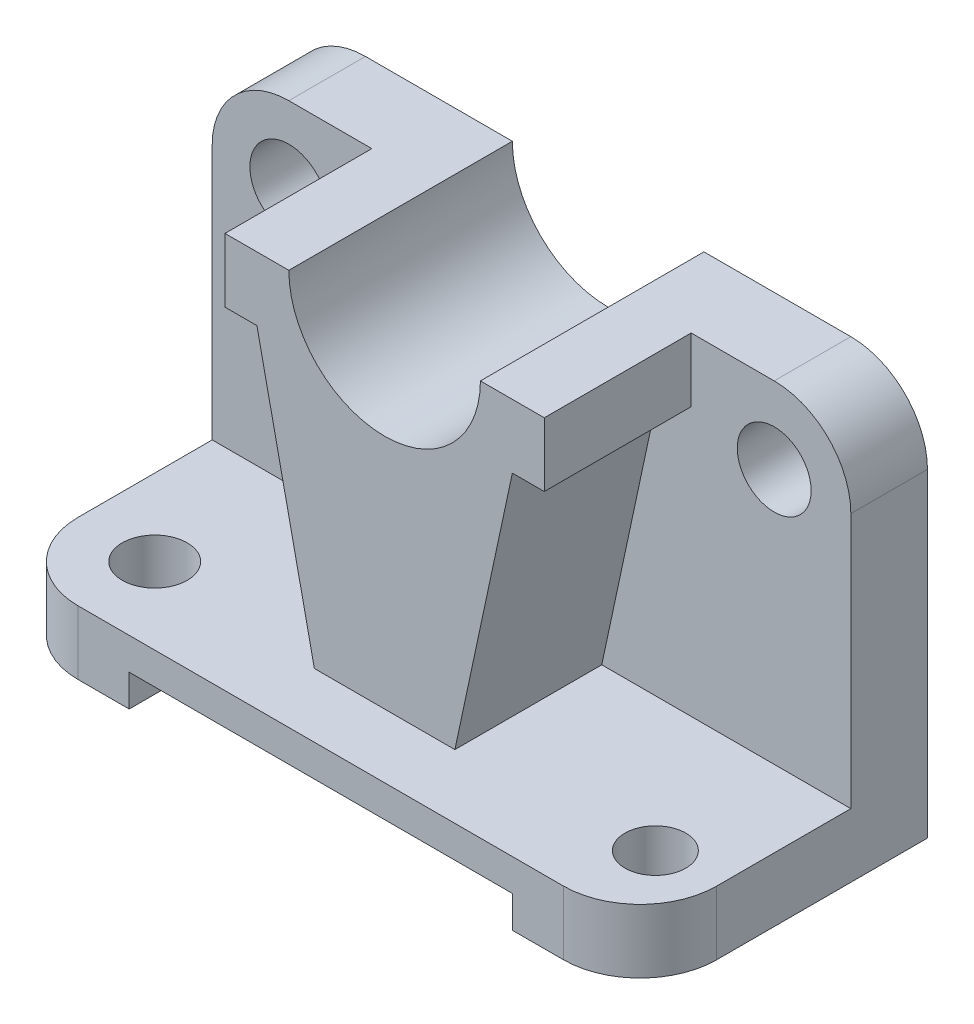
ISO-10303-21;
HEADER;
FILE_DESCRIPTION(('STEP AP214'),'2;1');
FILE_NAME('part.step','',(''),(''),'','','');
FILE_SCHEMA(('AUTOMOTIVE_DESIGN { 1 0 10303 214 1 1 1 1 }'));
ENDSEC;
DATA;
#1=APPLICATION_CONTEXT('core data for automotive mechanical design processes');
#2=APPLICATION_PROTOCOL_DEFINITION('international standard','automotive_design',2000,#1);
#3=PRODUCT_CONTEXT('',#1,'mechanical');
#4=PRODUCT('Part','Part','',(#3));
#5=PRODUCT_RELATED_PRODUCT_CATEGORY('part','',(#4));
#6=PRODUCT_DEFINITION_FORMATION('','',#4);
#7=PRODUCT_DEFINITION_CONTEXT('part definition',#1,'design');
#8=PRODUCT_DEFINITION('design','',#6,#7);
#9=PRODUCT_DEFINITION_SHAPE('','',#8);
#10=(LENGTH_UNIT() NAMED_UNIT(*) SI_UNIT(.MILLI.,.METRE.));
#11=(NAMED_UNIT(*) PLANE_ANGLE_UNIT() SI_UNIT($,.RADIAN.));
#12=(NAMED_UNIT(*) SI_UNIT($,.STERADIAN.) SOLID_ANGLE_UNIT());
#13=UNCERTAINTY_MEASURE_WITH_UNIT(LENGTH_MEASURE(1.E-05),#10,'distance_accuracy_value','');
#14=(GEOMETRIC_REPRESENTATION_CONTEXT(3) GLOBAL_UNCERTAINTY_ASSIGNED_CONTEXT((#13)) GLOBAL_UNIT_ASSIGNED_CONTEXT((#10,
#11,#12)) REPRESENTATION_CONTEXT('',''));
#15=CARTESIAN_POINT('',(0.,0.,0.));
#16=DIRECTION('',(0.,0.,1.));
#17=DIRECTION('',(1.,0.,0.));
#18=AXIS2_PLACEMENT_3D('',#15,#16,#17);
#19=CARTESIAN_POINT('',(0.,62.,-10.5));
#20=DIRECTION('',(0.,-1.,0.));
#21=DIRECTION('',(0.,0.,-1.));
#22=AXIS2_PLACEMENT_3D('',#19,#20,#21);
#23=PLANE('',#22);
#24=DIRECTION('',(1.,0.,0.));
#25=VECTOR('',#24,1.);
#26=CARTESIAN_POINT('',(0.,62.,-10.5));
#27=LINE('',#26,#25);
#28=CARTESIAN_POINT('',(75.,62.,-10.5));
#29=VERTEX_POINT('',#28);
#30=CARTESIAN_POINT('',(88.,62.,-10.5));
#31=VERTEX_POINT('',#30);
#32=EDGE_CURVE('E230',#29,#31,#27,.T.);
#33=ORIENTED_EDGE('',*,*,#32,.T.);
#34=DIRECTION('',(0.,0.,-1.));
#35=VECTOR('',#34,1.);
#36=CARTESIAN_POINT('',(88.,62.,-10.5));
#37=LINE('',#36,#35);
#38=CARTESIAN_POINT('',(88.,62.,-22.5));
#39=VERTEX_POINT('',#38);
#40=EDGE_CURVE('E50',#31,#39,#37,.T.);
#41=ORIENTED_EDGE('',*,*,#40,.T.);
#42=DIRECTION('',(1.,0.,0.));
#43=VECTOR('',#42,1.);
#44=CARTESIAN_POINT('',(0.,62.,-22.5));
#45=LINE('',#44,#43);
#46=CARTESIAN_POINT('',(65.,62.,-22.5));
#47=VERTEX_POINT('',#46);
#48=EDGE_CURVE('E217',#47,#39,#45,.T.);
#49=ORIENTED_EDGE('',*,*,#48,.F.);
#50=DIRECTION('',(0.,0.,-1.));
#51=VECTOR('',#50,1.);
#52=CARTESIAN_POINT('',(65.,62.,12.5));
#53=LINE('',#52,#51);
#54=CARTESIAN_POINT('',(65.,62.,12.5));
#55=VERTEX_POINT('',#54);
#56=EDGE_CURVE('E205',#55,#47,#53,.T.);
#57=ORIENTED_EDGE('',*,*,#56,.F.);
#58=DIRECTION('',(-1.,0.,0.));
#59=VECTOR('',#58,1.);
#60=CARTESIAN_POINT('',(75.,62.,12.5));
#61=LINE('',#60,#59);
#62=CARTESIAN_POINT('',(75.,62.,12.5));
#63=VERTEX_POINT('',#62);
#64=EDGE_CURVE('E456',#63,#55,#61,.T.);
#65=ORIENTED_EDGE('',*,*,#64,.F.);
#66=DIRECTION('',(0.,0.,-1.));
#67=VECTOR('',#66,1.);
#68=CARTESIAN_POINT('',(75.,62.,12.5));
#69=LINE('',#68,#67);
#70=EDGE_CURVE('E211',#63,#29,#69,.T.);
#71=ORIENTED_EDGE('',*,*,#70,.T.);
#72=EDGE_LOOP('',(#33,#41,#49,#57,#65,#71));
#73=FACE_BOUND('',#72,.T.);
#74=ADVANCED_FACE('F39',(#73),#23,.F.);
#75=CARTESIAN_POINT('',(100.,10.,22.5));
#76=DIRECTION('',(0.,-1.,0.));
#77=DIRECTION('',(0.,0.,-1.));
#78=AXIS2_PLACEMENT_3D('',#75,#76,#77);
#79=PLANE('',#78);
#80=CARTESIAN_POINT('',(12.,10.,10.5));
#81=DIRECTION('',(0.,1.,0.));
#82=DIRECTION('',(0.,0.,1.));
#83=AXIS2_PLACEMENT_3D('',#80,#81,#82);
#84=CIRCLE('',#83,5.09061435259613);
#85=CARTESIAN_POINT('',(12.,10.,15.5906143525961));
#86=VERTEX_POINT('',#85);
#87=EDGE_CURVE('E759',#86,#86,#84,.T.);
#88=ORIENTED_EDGE('',*,*,#87,.F.);
#89=EDGE_LOOP('',(#88));
#90=FACE_BOUND('',#89,.T.);
#91=CARTESIAN_POINT('',(90.3964880883435,10.,10.5));
#92=DIRECTION('',(0.,1.,0.));
#93=DIRECTION('',(0.,0.,1.));
#94=AXIS2_PLACEMENT_3D('',#91,#92,#93);
#95=CIRCLE('',#94,4.76218762017058);
#96=CARTESIAN_POINT('',(90.3964880883435,10.,15.2621876201706));
#97=VERTEX_POINT('',#96);
#98=EDGE_CURVE('E762',#97,#97,#95,.T.);
#99=ORIENTED_EDGE('',*,*,#98,.F.);
#100=EDGE_LOOP('',(#99));
#101=FACE_BOUND('',#100,.T.);
#102=DIRECTION('',(0.,0.,-1.));
#103=VECTOR('',#102,1.);
#104=CARTESIAN_POINT('',(0.,10.,22.5));
#105=LINE('',#104,#103);
#106=CARTESIAN_POINT('',(0.,10.,10.5));
#107=VERTEX_POINT('',#106);
#108=CARTESIAN_POINT('',(0.,10.,-10.5));
#109=VERTEX_POINT('',#108);
#110=EDGE_CURVE('E286',#107,#109,#105,.T.);
#111=ORIENTED_EDGE('',*,*,#110,.F.);
#112=CARTESIAN_POINT('',(12.,10.,10.5));
#113=DIRECTION('',(0.,-1.,0.));
#114=DIRECTION('',(0.,0.,-1.));
#115=AXIS2_PLACEMENT_3D('',#112,#113,#114);
#116=CIRCLE('',#115,12.);
#117=CARTESIAN_POINT('',(12.,10.,22.5));
#118=VERTEX_POINT('',#117);
#119=EDGE_CURVE('E308',#107,#118,#116,.F.);
#120=ORIENTED_EDGE('',*,*,#119,.T.);
#121=DIRECTION('',(-1.,0.,0.));
#122=VECTOR('',#121,1.);
#123=CARTESIAN_POINT('',(100.,10.,22.5));
#124=LINE('',#123,#122);
#125=CARTESIAN_POINT('',(88.,10.,22.5));
#126=VERTEX_POINT('',#125);
#127=EDGE_CURVE('E242',#126,#118,#124,.T.);
#128=ORIENTED_EDGE('',*,*,#127,.F.);
#129=CARTESIAN_POINT('',(88.,10.,10.5));
#130=DIRECTION('',(0.,-1.,0.));
#131=DIRECTION('',(0.,0.,-1.));
#132=AXIS2_PLACEMENT_3D('',#129,#130,#131);
#133=CIRCLE('',#132,12.);
#134=CARTESIAN_POINT('',(100.,10.,10.5));
#135=VERTEX_POINT('',#134);
#136=EDGE_CURVE('E303',#126,#135,#133,.F.);
#137=ORIENTED_EDGE('',*,*,#136,.T.);
#138=DIRECTION('',(0.,0.,-1.));
#139=VECTOR('',#138,1.);
#140=CARTESIAN_POINT('',(100.,10.,22.5));
#141=LINE('',#140,#139);
#142=CARTESIAN_POINT('',(100.,10.,-10.5));
#143=VERTEX_POINT('',#142);
#144=EDGE_CURVE('E288',#135,#143,#141,.T.);
#145=ORIENTED_EDGE('',*,*,#144,.T.);
#146=DIRECTION('',(1.,0.,0.));
#147=VECTOR('',#146,1.);
#148=CARTESIAN_POINT('',(0.,10.,-10.5));
#149=LINE('',#148,#147);
#150=CARTESIAN_POINT('',(61.,10.,-10.5));
#151=VERTEX_POINT('',#150);
#152=EDGE_CURVE('E237',#151,#143,#149,.T.);
#153=ORIENTED_EDGE('',*,*,#152,.F.);
#154=DIRECTION('',(0.,0.,-1.));
#155=VECTOR('',#154,1.);
#156=CARTESIAN_POINT('',(61.,10.,12.5));
#157=LINE('',#156,#155);
#158=CARTESIAN_POINT('',(61.,10.,12.5));
#159=VERTEX_POINT('',#158);
#160=EDGE_CURVE('E355',#159,#151,#157,.T.);
#161=ORIENTED_EDGE('',*,*,#160,.F.);
#162=DIRECTION('',(1.,0.,0.));
#163=VECTOR('',#162,1.);
#164=CARTESIAN_POINT('',(39.,10.,12.5));
#165=LINE('',#164,#163);
#166=CARTESIAN_POINT('',(39.,10.,12.5));
#167=VERTEX_POINT('',#166);
#168=EDGE_CURVE('E408',#167,#159,#165,.T.);
#169=ORIENTED_EDGE('',*,*,#168,.F.);
#170=DIRECTION('',(0.,0.,-1.));
#171=VECTOR('',#170,1.);
#172=CARTESIAN_POINT('',(39.,10.,12.5));
#173=LINE('',#172,#171);
#174=CARTESIAN_POINT('',(39.,10.,-10.5));
#175=VERTEX_POINT('',#174);
#176=EDGE_CURVE('E353',#167,#175,#173,.T.);
#177=ORIENTED_EDGE('',*,*,#176,.T.);
#178=EDGE_CURVE('E240',#109,#175,#149,.T.);
#179=ORIENTED_EDGE('',*,*,#178,.F.);
#180=EDGE_LOOP('',(#111,#120,#128,#137,#145,#153,#161,#169,#177,#179));
#181=FACE_BOUND('',#180,.T.);
#182=ADVANCED_FACE('F401',(#90,#101,#181),#79,.F.);
#183=CARTESIAN_POINT('',(0.,10.,-10.5));
#184=DIRECTION('',(0.,0.,-1.));
#185=DIRECTION('',(-1.,0.,0.));
#186=AXIS2_PLACEMENT_3D('',#183,#184,#185);
#187=PLANE('',#186);
#188=CARTESIAN_POINT('',(88.,50.,-10.5));
#189=DIRECTION('',(0.,0.,1.));
#190=DIRECTION('',(1.,0.,0.));
#191=AXIS2_PLACEMENT_3D('',#188,#189,#190);
#192=CIRCLE('',#191,5.78308621894568);
#193=CARTESIAN_POINT('',(93.7830862189457,50.,-10.5));
#194=VERTEX_POINT('',#193);
#195=EDGE_CURVE('E750',#194,#194,#192,.T.);
#196=ORIENTED_EDGE('',*,*,#195,.F.);
#197=EDGE_LOOP('',(#196));
#198=FACE_BOUND('',#197,.T.);
#199=DIRECTION('',(0.,1.,0.));
#200=VECTOR('',#199,1.);
#201=CARTESIAN_POINT('',(100.,10.,-10.5));
#202=LINE('',#201,#200);
#203=CARTESIAN_POINT('',(100.,50.,-10.5));
#204=VERTEX_POINT('',#203);
#205=EDGE_CURVE('E228',#143,#204,#202,.T.);
#206=ORIENTED_EDGE('',*,*,#205,.T.);
#207=CARTESIAN_POINT('',(88.,50.,-10.5));
#208=DIRECTION('',(0.,0.,-1.));
#209=DIRECTION('',(-1.,0.,0.));
#210=AXIS2_PLACEMENT_3D('',#207,#208,#209);
#211=CIRCLE('',#210,12.);
#212=EDGE_CURVE('E11',#204,#31,#211,.F.);
#213=ORIENTED_EDGE('',*,*,#212,.T.);
#214=ORIENTED_EDGE('',*,*,#32,.F.);
#215=DIRECTION('',(0.,1.,0.));
#216=VECTOR('',#215,1.);
#217=CARTESIAN_POINT('',(75.,52.,-10.5));
#218=LINE('',#217,#216);
#219=CARTESIAN_POINT('',(75.,52.,-10.5));
#220=VERTEX_POINT('',#219);
#221=EDGE_CURVE('E423',#220,#29,#218,.T.);
#222=ORIENTED_EDGE('',*,*,#221,.F.);
#223=DIRECTION('',(1.,0.,0.));
#224=VECTOR('',#223,1.);
#225=CARTESIAN_POINT('',(75.,52.,-10.5));
#226=LINE('',#225,#224);
#227=CARTESIAN_POINT('',(70.,52.,-10.5));
#228=VERTEX_POINT('',#227);
#229=EDGE_CURVE('E420',#228,#220,#226,.T.);
#230=ORIENTED_EDGE('',*,*,#229,.F.);
#231=DIRECTION('',(0.209529088730874,0.97780241407741,0.));
#232=VECTOR('',#231,1.);
#233=CARTESIAN_POINT('',(70.,52.,-10.5));
#234=LINE('',#233,#232);
#235=EDGE_CURVE('E412',#151,#228,#234,.T.);
#236=ORIENTED_EDGE('',*,*,#235,.F.);
#237=ORIENTED_EDGE('',*,*,#152,.T.);
#238=EDGE_LOOP('',(#206,#213,#214,#222,#230,#236,#237));
#239=FACE_BOUND('',#238,.T.);
#240=ADVANCED_FACE('F362',(#198,#239),#187,.F.);
#241=CARTESIAN_POINT('',(12.,50.,-10.5));
#242=DIRECTION('',(0.,0.,1.));
#243=DIRECTION('',(1.,0.,0.));
#244=AXIS2_PLACEMENT_3D('',#241,#242,#243);
#245=CIRCLE('',#244,6.102513624206);
#246=CARTESIAN_POINT('',(18.102513624206,50.,-10.5));
#247=VERTEX_POINT('',#246);
#248=EDGE_CURVE('E225',#247,#247,#245,.T.);
#249=ORIENTED_EDGE('',*,*,#248,.F.);
#250=EDGE_LOOP('',(#249));
#251=FACE_BOUND('',#250,.T.);
#252=CARTESIAN_POINT('',(12.,62.,-10.5));
#253=VERTEX_POINT('',#252);
#254=CARTESIAN_POINT('',(25.,62.,-10.5));
#255=VERTEX_POINT('',#254);
#256=EDGE_CURVE('E233',#253,#255,#27,.T.);
#257=ORIENTED_EDGE('',*,*,#256,.F.);
#258=CARTESIAN_POINT('',(12.,50.,-10.5));
#259=DIRECTION('',(0.,0.,-1.));
#260=DIRECTION('',(-1.,0.,0.));
#261=AXIS2_PLACEMENT_3D('',#258,#259,#260);
#262=CIRCLE('',#261,12.);
#263=CARTESIAN_POINT('',(0.,50.,-10.5));
#264=VERTEX_POINT('',#263);
#265=EDGE_CURVE('E317',#253,#264,#262,.F.);
#266=ORIENTED_EDGE('',*,*,#265,.T.);
#267=DIRECTION('',(0.,1.,0.));
#268=VECTOR('',#267,1.);
#269=CARTESIAN_POINT('',(0.,10.,-10.5));
#270=LINE('',#269,#268);
#271=EDGE_CURVE('E227',#109,#264,#270,.T.);
#272=ORIENTED_EDGE('',*,*,#271,.F.);
#273=ORIENTED_EDGE('',*,*,#178,.T.);
#274=DIRECTION('',(0.209529088730874,-0.977802414077409,0.));
#275=VECTOR('',#274,1.);
#276=CARTESIAN_POINT('',(30.,52.,-10.5));
#277=LINE('',#276,#275);
#278=CARTESIAN_POINT('',(30.,52.,-10.5));
#279=VERTEX_POINT('',#278);
#280=EDGE_CURVE('E222',#279,#175,#277,.T.);
#281=ORIENTED_EDGE('',*,*,#280,.F.);
#282=DIRECTION('',(1.,0.,0.));
#283=VECTOR('',#282,1.);
#284=CARTESIAN_POINT('',(25.,52.,-10.5));
#285=LINE('',#284,#283);
#286=CARTESIAN_POINT('',(25.,52.,-10.5));
#287=VERTEX_POINT('',#286);
#288=EDGE_CURVE('E427',#287,#279,#285,.T.);
#289=ORIENTED_EDGE('',*,*,#288,.F.);
#290=DIRECTION('',(0.,-1.,0.));
#291=VECTOR('',#290,1.);
#292=CARTESIAN_POINT('',(25.,62.,-10.5));
#293=LINE('',#292,#291);
#294=EDGE_CURVE('E430',#255,#287,#293,.T.);
#295=ORIENTED_EDGE('',*,*,#294,.F.);
#296=EDGE_LOOP('',(#257,#266,#272,#273,#281,#289,#295));
#297=FACE_BOUND('',#296,.T.);
#298=ADVANCED_FACE('F323',(#251,#297),#187,.F.);
#299=CARTESIAN_POINT('',(100.,0.,22.5));
#300=DIRECTION('',(-1.,0.,0.));
#301=DIRECTION('',(0.,0.,1.));
#302=AXIS2_PLACEMENT_3D('',#299,#300,#301);
#303=PLANE('',#302);
#304=ORIENTED_EDGE('',*,*,#144,.F.);
#305=DIRECTION('',(0.,1.,0.));
#306=VECTOR('',#305,1.);
#307=CARTESIAN_POINT('',(100.,0.,10.5));
#308=LINE('',#307,#306);
#309=CARTESIAN_POINT('',(100.,0.,10.5));
#310=VERTEX_POINT('',#309);
#311=EDGE_CURVE('E309',#135,#310,#308,.F.);
#312=ORIENTED_EDGE('',*,*,#311,.T.);
#313=DIRECTION('',(0.,0.,-1.));
#314=VECTOR('',#313,1.);
#315=CARTESIAN_POINT('',(100.,0.,22.5));
#316=LINE('',#315,#314);
#317=CARTESIAN_POINT('',(100.,0.,-22.5));
#318=VERTEX_POINT('',#317);
#319=EDGE_CURVE('E258',#310,#318,#316,.T.);
#320=ORIENTED_EDGE('',*,*,#319,.T.);
#321=DIRECTION('',(0.,1.,0.));
#322=VECTOR('',#321,1.);
#323=CARTESIAN_POINT('',(100.,0.,-22.5));
#324=LINE('',#323,#322);
#325=CARTESIAN_POINT('',(100.,50.,-22.5));
#326=VERTEX_POINT('',#325);
#327=EDGE_CURVE('E238',#318,#326,#324,.T.);
#328=ORIENTED_EDGE('',*,*,#327,.T.);
#329=DIRECTION('',(0.,0.,-1.));
#330=VECTOR('',#329,1.);
#331=CARTESIAN_POINT('',(100.,50.,22.5));
#332=LINE('',#331,#330);
#333=EDGE_CURVE('E306',#326,#204,#332,.F.);
#334=ORIENTED_EDGE('',*,*,#333,.T.);
#335=ORIENTED_EDGE('',*,*,#205,.F.);
#336=EDGE_LOOP('',(#304,#312,#320,#328,#334,#335));
#337=FACE_BOUND('',#336,.T.);
#338=ADVANCED_FACE('F371',(#337),#303,.F.);
#339=CARTESIAN_POINT('',(0.,10.,22.5));
#340=DIRECTION('',(1.,0.,0.));
#341=DIRECTION('',(0.,0.,-1.));
#342=AXIS2_PLACEMENT_3D('',#339,#340,#341);
#343=PLANE('',#342);
#344=DIRECTION('',(0.,0.,-1.));
#345=VECTOR('',#344,1.);
#346=CARTESIAN_POINT('',(0.,0.,22.5));
#347=LINE('',#346,#345);
#348=CARTESIAN_POINT('',(0.,0.,10.5));
#349=VERTEX_POINT('',#348);
#350=CARTESIAN_POINT('',(0.,0.,-22.5));
#351=VERTEX_POINT('',#350);
#352=EDGE_CURVE('E281',#349,#351,#347,.T.);
#353=ORIENTED_EDGE('',*,*,#352,.F.);
#354=DIRECTION('',(0.,-1.,0.));
#355=VECTOR('',#354,1.);
#356=CARTESIAN_POINT('',(0.,10.,10.5));
#357=LINE('',#356,#355);
#358=EDGE_CURVE('E301',#349,#107,#357,.F.);
#359=ORIENTED_EDGE('',*,*,#358,.T.);
#360=ORIENTED_EDGE('',*,*,#110,.T.);
#361=ORIENTED_EDGE('',*,*,#271,.T.);
#362=DIRECTION('',(0.,0.,-1.));
#363=VECTOR('',#362,1.);
#364=CARTESIAN_POINT('',(0.,50.,22.5));
#365=LINE('',#364,#363);
#366=CARTESIAN_POINT('',(0.,50.,-22.5));
#367=VERTEX_POINT('',#366);
#368=EDGE_CURVE('E296',#264,#367,#365,.T.);
#369=ORIENTED_EDGE('',*,*,#368,.T.);
#370=DIRECTION('',(0.,-1.,0.));
#371=VECTOR('',#370,1.);
#372=CARTESIAN_POINT('',(0.,10.,-22.5));
#373=LINE('',#372,#371);
#374=EDGE_CURVE('E259',#367,#351,#373,.T.);
#375=ORIENTED_EDGE('',*,*,#374,.T.);
#376=EDGE_LOOP('',(#353,#359,#360,#361,#369,#375));
#377=FACE_BOUND('',#376,.T.);
#378=ADVANCED_FACE('F328',(#377),#343,.F.);
#379=CARTESIAN_POINT('',(0.,0.,22.5));
#380=DIRECTION('',(0.,1.,0.));
#381=DIRECTION('',(0.,0.,1.));
#382=AXIS2_PLACEMENT_3D('',#379,#380,#381);
#383=PLANE('',#382);
#384=CARTESIAN_POINT('',(12.,0.,10.5));
#385=DIRECTION('',(0.,1.,0.));
#386=DIRECTION('',(0.,0.,1.));
#387=AXIS2_PLACEMENT_3D('',#384,#385,#386);
#388=CIRCLE('',#387,5.09061435259613);
#389=CARTESIAN_POINT('',(12.,0.,15.5906143525961));
#390=VERTEX_POINT('',#389);
#391=EDGE_CURVE('E760',#390,#390,#388,.T.);
#392=ORIENTED_EDGE('',*,*,#391,.T.);
#393=EDGE_LOOP('',(#392));
#394=FACE_BOUND('',#393,.T.);
#395=DIRECTION('',(1.,0.,0.));
#396=VECTOR('',#395,1.);
#397=CARTESIAN_POINT('',(0.,0.,22.5));
#398=LINE('',#397,#396);
#399=CARTESIAN_POINT('',(12.,0.,22.5));
#400=VERTEX_POINT('',#399);
#401=CARTESIAN_POINT('',(20.,0.,22.5));
#402=VERTEX_POINT('',#401);
#403=EDGE_CURVE('E241',#400,#402,#398,.T.);
#404=ORIENTED_EDGE('',*,*,#403,.F.);
#405=CARTESIAN_POINT('',(12.,0.,10.5));
#406=DIRECTION('',(0.,1.,0.));
#407=DIRECTION('',(0.,0.,1.));
#408=AXIS2_PLACEMENT_3D('',#405,#406,#407);
#409=CIRCLE('',#408,12.);
#410=EDGE_CURVE('E299',#400,#349,#409,.F.);
#411=ORIENTED_EDGE('',*,*,#410,.T.);
#412=ORIENTED_EDGE('',*,*,#352,.T.);
#413=DIRECTION('',(1.,0.,0.));
#414=VECTOR('',#413,1.);
#415=CARTESIAN_POINT('',(0.,0.,-22.5));
#416=LINE('',#415,#414);
#417=CARTESIAN_POINT('',(20.,0.,-22.5));
#418=VERTEX_POINT('',#417);
#419=EDGE_CURVE('E261',#351,#418,#416,.T.);
#420=ORIENTED_EDGE('',*,*,#419,.T.);
#421=DIRECTION('',(0.,0.,-1.));
#422=VECTOR('',#421,1.);
#423=CARTESIAN_POINT('',(20.,0.,22.5));
#424=LINE('',#423,#422);
#425=EDGE_CURVE('E282',#402,#418,#424,.T.);
#426=ORIENTED_EDGE('',*,*,#425,.F.);
#427=EDGE_LOOP('',(#404,#411,#412,#420,#426));
#428=FACE_BOUND('',#427,.T.);
#429=ADVANCED_FACE('F399',(#394,#428),#383,.F.);
#430=CARTESIAN_POINT('',(20.,0.,22.5));
#431=DIRECTION('',(-1.,0.,0.));
#432=DIRECTION('',(0.,0.,1.));
#433=AXIS2_PLACEMENT_3D('',#430,#431,#432);
#434=PLANE('',#433);
#435=DIRECTION('',(0.,1.,0.));
#436=VECTOR('',#435,1.);
#437=CARTESIAN_POINT('',(20.,0.,-22.5));
#438=LINE('',#437,#436);
#439=CARTESIAN_POINT('',(20.,5.,-22.5));
#440=VERTEX_POINT('',#439);
#441=EDGE_CURVE('E263',#418,#440,#438,.T.);
#442=ORIENTED_EDGE('',*,*,#441,.T.);
#443=DIRECTION('',(0.,0.,-1.));
#444=VECTOR('',#443,1.);
#445=CARTESIAN_POINT('',(20.,5.,22.5));
#446=LINE('',#445,#444);
#447=CARTESIAN_POINT('',(20.,5.,22.5));
#448=VERTEX_POINT('',#447);
#449=EDGE_CURVE('E279',#448,#440,#446,.T.);
#450=ORIENTED_EDGE('',*,*,#449,.F.);
#451=DIRECTION('',(0.,1.,0.));
#452=VECTOR('',#451,1.);
#453=CARTESIAN_POINT('',(20.,0.,22.5));
#454=LINE('',#453,#452);
#455=EDGE_CURVE('E246',#402,#448,#454,.T.);
#456=ORIENTED_EDGE('',*,*,#455,.F.);
#457=ORIENTED_EDGE('',*,*,#425,.T.);
#458=EDGE_LOOP('',(#442,#450,#456,#457));
#459=FACE_BOUND('',#458,.T.);
#460=ADVANCED_FACE('F394',(#459),#434,.F.);
#461=CARTESIAN_POINT('',(20.,5.,22.5));
#462=DIRECTION('',(0.,1.,0.));
#463=DIRECTION('',(0.,0.,1.));
#464=AXIS2_PLACEMENT_3D('',#461,#462,#463);
#465=PLANE('',#464);
#466=DIRECTION('',(1.,0.,0.));
#467=VECTOR('',#466,1.);
#468=CARTESIAN_POINT('',(20.,5.,-22.5));
#469=LINE('',#468,#467);
#470=CARTESIAN_POINT('',(80.,5.,-22.5));
#471=VERTEX_POINT('',#470);
#472=EDGE_CURVE('E264',#440,#471,#469,.T.);
#473=ORIENTED_EDGE('',*,*,#472,.T.);
#474=DIRECTION('',(0.,0.,-1.));
#475=VECTOR('',#474,1.);
#476=CARTESIAN_POINT('',(80.,5.,22.5));
#477=LINE('',#476,#475);
#478=CARTESIAN_POINT('',(80.,5.,22.5));
#479=VERTEX_POINT('',#478);
#480=EDGE_CURVE('E274',#479,#471,#477,.T.);
#481=ORIENTED_EDGE('',*,*,#480,.F.);
#482=DIRECTION('',(1.,0.,0.));
#483=VECTOR('',#482,1.);
#484=CARTESIAN_POINT('',(20.,5.,22.5));
#485=LINE('',#484,#483);
#486=EDGE_CURVE('E248',#448,#479,#485,.T.);
#487=ORIENTED_EDGE('',*,*,#486,.F.);
#488=ORIENTED_EDGE('',*,*,#449,.T.);
#489=EDGE_LOOP('',(#473,#481,#487,#488));
#490=FACE_BOUND('',#489,.T.);
#491=ADVANCED_FACE('F389',(#490),#465,.F.);
#492=CARTESIAN_POINT('',(80.,5.,22.5));
#493=DIRECTION('',(1.,0.,0.));
#494=DIRECTION('',(0.,0.,-1.));
#495=AXIS2_PLACEMENT_3D('',#492,#493,#494);
#496=PLANE('',#495);
#497=DIRECTION('',(0.,-1.,0.));
#498=VECTOR('',#497,1.);
#499=CARTESIAN_POINT('',(80.,5.,-22.5));
#500=LINE('',#499,#498);
#501=CARTESIAN_POINT('',(80.,0.,-22.5));
#502=VERTEX_POINT('',#501);
#503=EDGE_CURVE('E270',#471,#502,#500,.T.);
#504=ORIENTED_EDGE('',*,*,#503,.T.);
#505=DIRECTION('',(0.,0.,-1.));
#506=VECTOR('',#505,1.);
#507=CARTESIAN_POINT('',(80.,0.,22.5));
#508=LINE('',#507,#506);
#509=CARTESIAN_POINT('',(80.,0.,22.5));
#510=VERTEX_POINT('',#509);
#511=EDGE_CURVE('E275',#510,#502,#508,.T.);
#512=ORIENTED_EDGE('',*,*,#511,.F.);
#513=DIRECTION('',(0.,-1.,0.));
#514=VECTOR('',#513,1.);
#515=CARTESIAN_POINT('',(80.,5.,22.5));
#516=LINE('',#515,#514);
#517=EDGE_CURVE('E253',#479,#510,#516,.T.);
#518=ORIENTED_EDGE('',*,*,#517,.F.);
#519=ORIENTED_EDGE('',*,*,#480,.T.);
#520=EDGE_LOOP('',(#504,#512,#518,#519));
#521=FACE_BOUND('',#520,.T.);
#522=ADVANCED_FACE('F382',(#521),#496,.F.);
#523=CARTESIAN_POINT('',(80.,0.,22.5));
#524=DIRECTION('',(0.,1.,0.));
#525=DIRECTION('',(0.,0.,1.));
#526=AXIS2_PLACEMENT_3D('',#523,#524,#525);
#527=PLANE('',#526);
#528=CARTESIAN_POINT('',(90.3964880883435,0.,10.5));
#529=DIRECTION('',(0.,1.,0.));
#530=DIRECTION('',(0.,0.,1.));
#531=AXIS2_PLACEMENT_3D('',#528,#529,#530);
#532=CIRCLE('',#531,4.76218762017058);
#533=CARTESIAN_POINT('',(90.3964880883435,0.,15.2621876201706));
#534=VERTEX_POINT('',#533);
#535=EDGE_CURVE('E755',#534,#534,#532,.T.);
#536=ORIENTED_EDGE('',*,*,#535,.T.);
#537=EDGE_LOOP('',(#536));
#538=FACE_BOUND('',#537,.T.);
#539=ORIENTED_EDGE('',*,*,#319,.F.);
#540=CARTESIAN_POINT('',(88.,0.,10.5));
#541=DIRECTION('',(0.,1.,0.));
#542=DIRECTION('',(0.,0.,1.));
#543=AXIS2_PLACEMENT_3D('',#540,#541,#542);
#544=CIRCLE('',#543,12.);
#545=CARTESIAN_POINT('',(88.,0.,22.5));
#546=VERTEX_POINT('',#545);
#547=EDGE_CURVE('E315',#310,#546,#544,.F.);
#548=ORIENTED_EDGE('',*,*,#547,.T.);
#549=DIRECTION('',(1.,0.,0.));
#550=VECTOR('',#549,1.);
#551=CARTESIAN_POINT('',(80.,0.,22.5));
#552=LINE('',#551,#550);
#553=EDGE_CURVE('E251',#510,#546,#552,.T.);
#554=ORIENTED_EDGE('',*,*,#553,.F.);
#555=ORIENTED_EDGE('',*,*,#511,.T.);
#556=DIRECTION('',(1.,0.,0.));
#557=VECTOR('',#556,1.);
#558=CARTESIAN_POINT('',(80.,0.,-22.5));
#559=LINE('',#558,#557);
#560=EDGE_CURVE('E243',#502,#318,#559,.T.);
#561=ORIENTED_EDGE('',*,*,#560,.T.);
#562=EDGE_LOOP('',(#539,#548,#554,#555,#561));
#563=FACE_BOUND('',#562,.T.);
#564=ADVANCED_FACE('F376',(#538,#563),#527,.F.);
#565=CARTESIAN_POINT('',(0.,0.,22.5));
#566=DIRECTION('',(0.,0.,1.));
#567=DIRECTION('',(1.,0.,0.));
#568=AXIS2_PLACEMENT_3D('',#565,#566,#567);
#569=PLANE('',#568);
#570=ORIENTED_EDGE('',*,*,#127,.T.);
#571=DIRECTION('',(0.,-1.,0.));
#572=VECTOR('',#571,1.);
#573=CARTESIAN_POINT('',(12.,0.,22.5));
#574=LINE('',#573,#572);
#575=EDGE_CURVE('E294',#118,#400,#574,.T.);
#576=ORIENTED_EDGE('',*,*,#575,.T.);
#577=ORIENTED_EDGE('',*,*,#403,.T.);
#578=ORIENTED_EDGE('',*,*,#455,.T.);
#579=ORIENTED_EDGE('',*,*,#486,.T.);
#580=ORIENTED_EDGE('',*,*,#517,.T.);
#581=ORIENTED_EDGE('',*,*,#553,.T.);
#582=DIRECTION('',(0.,1.,0.));
#583=VECTOR('',#582,1.);
#584=CARTESIAN_POINT('',(88.,10.,22.5));
#585=LINE('',#584,#583);
#586=EDGE_CURVE('E292',#546,#126,#585,.T.);
#587=ORIENTED_EDGE('',*,*,#586,.T.);
#588=EDGE_LOOP('',(#570,#576,#577,#578,#579,#580,#581,#587));
#589=FACE_BOUND('',#588,.T.);
#590=ADVANCED_FACE('F403',(#589),#569,.T.);
#591=CARTESIAN_POINT('',(0.,0.,-22.5));
#592=DIRECTION('',(0.,0.,1.));
#593=DIRECTION('',(1.,0.,0.));
#594=AXIS2_PLACEMENT_3D('',#591,#592,#593);
#595=PLANE('',#594);
#596=CARTESIAN_POINT('',(88.,50.,-22.5));
#597=DIRECTION('',(0.,0.,1.));
#598=DIRECTION('',(1.,0.,0.));
#599=AXIS2_PLACEMENT_3D('',#596,#597,#598);
#600=CIRCLE('',#599,5.78308621894568);
#601=CARTESIAN_POINT('',(93.7830862189457,50.,-22.5));
#602=VERTEX_POINT('',#601);
#603=EDGE_CURVE('E756',#602,#602,#600,.T.);
#604=ORIENTED_EDGE('',*,*,#603,.T.);
#605=EDGE_LOOP('',(#604));
#606=FACE_BOUND('',#605,.T.);
#607=CARTESIAN_POINT('',(12.,50.,-22.5));
#608=DIRECTION('',(0.,0.,1.));
#609=DIRECTION('',(1.,0.,0.));
#610=AXIS2_PLACEMENT_3D('',#607,#608,#609);
#611=CIRCLE('',#610,6.102513624206);
#612=CARTESIAN_POINT('',(18.102513624206,50.,-22.5));
#613=VERTEX_POINT('',#612);
#614=EDGE_CURVE('E748',#613,#613,#611,.T.);
#615=ORIENTED_EDGE('',*,*,#614,.T.);
#616=EDGE_LOOP('',(#615));
#617=FACE_BOUND('',#616,.T.);
#618=ORIENTED_EDGE('',*,*,#374,.F.);
#619=CARTESIAN_POINT('',(12.,50.,-22.5));
#620=DIRECTION('',(0.,0.,1.));
#621=DIRECTION('',(1.,0.,0.));
#622=AXIS2_PLACEMENT_3D('',#619,#620,#621);
#623=CIRCLE('',#622,12.);
#624=CARTESIAN_POINT('',(12.,62.,-22.5));
#625=VERTEX_POINT('',#624);
#626=EDGE_CURVE('E316',#367,#625,#623,.F.);
#627=ORIENTED_EDGE('',*,*,#626,.T.);
#628=CARTESIAN_POINT('',(35.,62.,-22.5));
#629=VERTEX_POINT('',#628);
#630=EDGE_CURVE('E218',#625,#629,#45,.T.);
#631=ORIENTED_EDGE('',*,*,#630,.T.);
#632=CARTESIAN_POINT('',(50.,62.,-22.5));
#633=DIRECTION('',(0.,0.,1.));
#634=DIRECTION('',(1.,0.,0.));
#635=AXIS2_PLACEMENT_3D('',#632,#633,#634);
#636=CIRCLE('',#635,15.);
#637=EDGE_CURVE('E206',#629,#47,#636,.T.);
#638=ORIENTED_EDGE('',*,*,#637,.T.);
#639=ORIENTED_EDGE('',*,*,#48,.T.);
#640=CARTESIAN_POINT('',(88.,50.,-22.5));
#641=DIRECTION('',(0.,0.,1.));
#642=DIRECTION('',(1.,0.,0.));
#643=AXIS2_PLACEMENT_3D('',#640,#641,#642);
#644=CIRCLE('',#643,12.);
#645=EDGE_CURVE('E314',#39,#326,#644,.F.);
#646=ORIENTED_EDGE('',*,*,#645,.T.);
#647=ORIENTED_EDGE('',*,*,#327,.F.);
#648=ORIENTED_EDGE('',*,*,#560,.F.);
#649=ORIENTED_EDGE('',*,*,#503,.F.);
#650=ORIENTED_EDGE('',*,*,#472,.F.);
#651=ORIENTED_EDGE('',*,*,#441,.F.);
#652=ORIENTED_EDGE('',*,*,#419,.F.);
#653=EDGE_LOOP('',(#618,#627,#631,#638,#639,#646,#647,#648,#649,#650,#651,#652));
#654=FACE_BOUND('',#653,.T.);
#655=ADVANCED_FACE('F220',(#606,#617,#654),#595,.F.);
#656=ORIENTED_EDGE('',*,*,#630,.F.);
#657=DIRECTION('',(0.,0.,-1.));
#658=VECTOR('',#657,1.);
#659=CARTESIAN_POINT('',(12.,62.,-10.5));
#660=LINE('',#659,#658);
#661=EDGE_CURVE('E58',#625,#253,#660,.F.);
#662=ORIENTED_EDGE('',*,*,#661,.T.);
#663=ORIENTED_EDGE('',*,*,#256,.T.);
#664=DIRECTION('',(0.,0.,-1.));
#665=VECTOR('',#664,1.);
#666=CARTESIAN_POINT('',(25.,62.,12.5));
#667=LINE('',#666,#665);
#668=CARTESIAN_POINT('',(25.,62.,12.5));
#669=VERTEX_POINT('',#668);
#670=EDGE_CURVE('E340',#669,#255,#667,.T.);
#671=ORIENTED_EDGE('',*,*,#670,.F.);
#672=DIRECTION('',(-1.,0.,0.));
#673=VECTOR('',#672,1.);
#674=CARTESIAN_POINT('',(35.,62.,12.5));
#675=LINE('',#674,#673);
#676=CARTESIAN_POINT('',(35.,62.,12.5));
#677=VERTEX_POINT('',#676);
#678=EDGE_CURVE('E339',#677,#669,#675,.T.);
#679=ORIENTED_EDGE('',*,*,#678,.F.);
#680=DIRECTION('',(0.,0.,-1.));
#681=VECTOR('',#680,1.);
#682=CARTESIAN_POINT('',(35.,62.,12.5));
#683=LINE('',#682,#681);
#684=EDGE_CURVE('E215',#677,#629,#683,.T.);
#685=ORIENTED_EDGE('',*,*,#684,.T.);
#686=EDGE_LOOP('',(#656,#662,#663,#671,#679,#685));
#687=FACE_BOUND('',#686,.T.);
#688=ADVANCED_FACE('F331',(#687),#23,.F.);
#689=CARTESIAN_POINT('',(30.,52.,12.5));
#690=DIRECTION('',(0.977802414077409,0.209529088730874,0.));
#691=DIRECTION('',(-0.209529088730874,0.977802414077409,0.));
#692=AXIS2_PLACEMENT_3D('',#689,#690,#691);
#693=PLANE('',#692);
#694=ORIENTED_EDGE('',*,*,#280,.T.);
#695=ORIENTED_EDGE('',*,*,#176,.F.);
#696=DIRECTION('',(0.209529088730874,-0.977802414077409,0.));
#697=VECTOR('',#696,1.);
#698=CARTESIAN_POINT('',(30.,52.,12.5));
#699=LINE('',#698,#697);
#700=CARTESIAN_POINT('',(30.,52.,12.5));
#701=VERTEX_POINT('',#700);
#702=EDGE_CURVE('E431',#701,#167,#699,.T.);
#703=ORIENTED_EDGE('',*,*,#702,.F.);
#704=DIRECTION('',(0.,0.,-1.));
#705=VECTOR('',#704,1.);
#706=CARTESIAN_POINT('',(30.,52.,12.5));
#707=LINE('',#706,#705);
#708=EDGE_CURVE('E435',#701,#279,#707,.T.);
#709=ORIENTED_EDGE('',*,*,#708,.T.);
#710=EDGE_LOOP('',(#694,#695,#703,#709));
#711=FACE_BOUND('',#710,.T.);
#712=ADVANCED_FACE('F447',(#711),#693,.F.);
#713=CARTESIAN_POINT('',(70.,52.,12.5));
#714=DIRECTION('',(-0.977802414077409,0.209529088730874,0.));
#715=DIRECTION('',(-0.209529088730874,-0.97780241407741,0.));
#716=AXIS2_PLACEMENT_3D('',#713,#714,#715);
#717=PLANE('',#716);
#718=ORIENTED_EDGE('',*,*,#235,.T.);
#719=DIRECTION('',(0.,0.,-1.));
#720=VECTOR('',#719,1.);
#721=CARTESIAN_POINT('',(70.,52.,12.5));
#722=LINE('',#721,#720);
#723=CARTESIAN_POINT('',(70.,52.,12.5));
#724=VERTEX_POINT('',#723);
#725=EDGE_CURVE('E348',#724,#228,#722,.T.);
#726=ORIENTED_EDGE('',*,*,#725,.F.);
#727=DIRECTION('',(0.209529088730874,0.97780241407741,0.));
#728=VECTOR('',#727,1.);
#729=CARTESIAN_POINT('',(70.,52.,12.5));
#730=LINE('',#729,#728);
#731=EDGE_CURVE('E418',#159,#724,#730,.T.);
#732=ORIENTED_EDGE('',*,*,#731,.F.);
#733=ORIENTED_EDGE('',*,*,#160,.T.);
#734=EDGE_LOOP('',(#718,#726,#732,#733));
#735=FACE_BOUND('',#734,.T.);
#736=ADVANCED_FACE('F415',(#735),#717,.F.);
#737=CARTESIAN_POINT('',(75.,52.,12.5));
#738=DIRECTION('',(0.,1.,0.));
#739=DIRECTION('',(0.,0.,1.));
#740=AXIS2_PLACEMENT_3D('',#737,#738,#739);
#741=PLANE('',#740);
#742=ORIENTED_EDGE('',*,*,#229,.T.);
#743=DIRECTION('',(0.,0.,-1.));
#744=VECTOR('',#743,1.);
#745=CARTESIAN_POINT('',(75.,52.,12.5));
#746=LINE('',#745,#744);
#747=CARTESIAN_POINT('',(75.,52.,12.5));
#748=VERTEX_POINT('',#747);
#749=EDGE_CURVE('E350',#748,#220,#746,.T.);
#750=ORIENTED_EDGE('',*,*,#749,.F.);
#751=DIRECTION('',(1.,0.,0.));
#752=VECTOR('',#751,1.);
#753=CARTESIAN_POINT('',(75.,52.,12.5));
#754=LINE('',#753,#752);
#755=EDGE_CURVE('E453',#724,#748,#754,.T.);
#756=ORIENTED_EDGE('',*,*,#755,.F.);
#757=ORIENTED_EDGE('',*,*,#725,.T.);
#758=EDGE_LOOP('',(#742,#750,#756,#757));
#759=FACE_BOUND('',#758,.T.);
#760=ADVANCED_FACE('F621',(#759),#741,.F.);
#761=CARTESIAN_POINT('',(75.,52.,12.5));
#762=DIRECTION('',(-1.,0.,0.));
#763=DIRECTION('',(0.,0.,1.));
#764=AXIS2_PLACEMENT_3D('',#761,#762,#763);
#765=PLANE('',#764);
#766=ORIENTED_EDGE('',*,*,#221,.T.);
#767=ORIENTED_EDGE('',*,*,#70,.F.);
#768=DIRECTION('',(0.,1.,0.));
#769=VECTOR('',#768,1.);
#770=CARTESIAN_POINT('',(75.,52.,12.5));
#771=LINE('',#770,#769);
#772=EDGE_CURVE('E457',#748,#63,#771,.T.);
#773=ORIENTED_EDGE('',*,*,#772,.F.);
#774=ORIENTED_EDGE('',*,*,#749,.T.);
#775=EDGE_LOOP('',(#766,#767,#773,#774));
#776=FACE_BOUND('',#775,.T.);
#777=ADVANCED_FACE('F471',(#776),#765,.F.);
#778=CARTESIAN_POINT('',(50.,62.,12.5));
#779=DIRECTION('',(0.,0.,-1.));
#780=DIRECTION('',(-1.,0.,0.));
#781=AXIS2_PLACEMENT_3D('',#778,#779,#780);
#782=CYLINDRICAL_SURFACE('',#781,15.);
#783=ORIENTED_EDGE('',*,*,#56,.T.);
#784=ORIENTED_EDGE('',*,*,#637,.F.);
#785=ORIENTED_EDGE('',*,*,#684,.F.);
#786=CARTESIAN_POINT('',(50.,62.,12.5));
#787=DIRECTION('',(0.,0.,-1.));
#788=DIRECTION('',(1.,0.,0.));
#789=AXIS2_PLACEMENT_3D('',#786,#787,#788);
#790=CIRCLE('',#789,15.);
#791=EDGE_CURVE('E210',#55,#677,#790,.T.);
#792=ORIENTED_EDGE('',*,*,#791,.F.);
#793=EDGE_LOOP('',(#783,#784,#785,#792));
#794=FACE_BOUND('',#793,.T.);
#795=ADVANCED_FACE('F204',(#794),#782,.F.);
#796=CARTESIAN_POINT('',(25.,62.,12.5));
#797=DIRECTION('',(1.,0.,0.));
#798=DIRECTION('',(0.,1.,0.));
#799=AXIS2_PLACEMENT_3D('',#796,#797,#798);
#800=PLANE('',#799);
#801=ORIENTED_EDGE('',*,*,#294,.T.);
#802=DIRECTION('',(0.,0.,-1.));
#803=VECTOR('',#802,1.);
#804=CARTESIAN_POINT('',(25.,52.,12.5));
#805=LINE('',#804,#803);
#806=CARTESIAN_POINT('',(25.,52.,12.5));
#807=VERTEX_POINT('',#806);
#808=EDGE_CURVE('E344',#807,#287,#805,.T.);
#809=ORIENTED_EDGE('',*,*,#808,.F.);
#810=DIRECTION('',(0.,-1.,0.));
#811=VECTOR('',#810,1.);
#812=CARTESIAN_POINT('',(25.,62.,12.5));
#813=LINE('',#812,#811);
#814=EDGE_CURVE('E464',#669,#807,#813,.T.);
#815=ORIENTED_EDGE('',*,*,#814,.F.);
#816=ORIENTED_EDGE('',*,*,#670,.T.);
#817=EDGE_LOOP('',(#801,#809,#815,#816));
#818=FACE_BOUND('',#817,.T.);
#819=ADVANCED_FACE('F461',(#818),#800,.F.);
#820=CARTESIAN_POINT('',(25.,52.,12.5));
#821=DIRECTION('',(0.,1.,0.));
#822=DIRECTION('',(-1.,0.,0.));
#823=AXIS2_PLACEMENT_3D('',#820,#821,#822);
#824=PLANE('',#823);
#825=ORIENTED_EDGE('',*,*,#288,.T.);
#826=ORIENTED_EDGE('',*,*,#708,.F.);
#827=DIRECTION('',(1.,0.,0.));
#828=VECTOR('',#827,1.);
#829=CARTESIAN_POINT('',(25.,52.,12.5));
#830=LINE('',#829,#828);
#831=EDGE_CURVE('E432',#807,#701,#830,.T.);
#832=ORIENTED_EDGE('',*,*,#831,.F.);
#833=ORIENTED_EDGE('',*,*,#808,.T.);
#834=EDGE_LOOP('',(#825,#826,#832,#833));
#835=FACE_BOUND('',#834,.T.);
#836=ADVANCED_FACE('F439',(#835),#824,.F.);
#837=CARTESIAN_POINT('',(50.,62.,12.5));
#838=DIRECTION('',(0.,0.,1.));
#839=DIRECTION('',(1.,0.,0.));
#840=AXIS2_PLACEMENT_3D('',#837,#838,#839);
#841=PLANE('',#840);
#842=ORIENTED_EDGE('',*,*,#702,.T.);
#843=ORIENTED_EDGE('',*,*,#168,.T.);
#844=ORIENTED_EDGE('',*,*,#731,.T.);
#845=ORIENTED_EDGE('',*,*,#755,.T.);
#846=ORIENTED_EDGE('',*,*,#772,.T.);
#847=ORIENTED_EDGE('',*,*,#64,.T.);
#848=ORIENTED_EDGE('',*,*,#791,.T.);
#849=ORIENTED_EDGE('',*,*,#678,.T.);
#850=ORIENTED_EDGE('',*,*,#814,.T.);
#851=ORIENTED_EDGE('',*,*,#831,.T.);
#852=EDGE_LOOP('',(#842,#843,#844,#845,#846,#847,#848,#849,#850,#851));
#853=FACE_BOUND('',#852,.T.);
#854=ADVANCED_FACE('F465',(#853),#841,.T.);
#855=CARTESIAN_POINT('',(12.,50.,-22.5));
#856=DIRECTION('',(0.,0.,1.));
#857=DIRECTION('',(1.,0.,0.));
#858=AXIS2_PLACEMENT_3D('',#855,#856,#857);
#859=CYLINDRICAL_SURFACE('',#858,6.102513624206);
#860=ORIENTED_EDGE('',*,*,#614,.F.);
#861=EDGE_LOOP('',(#860));
#862=FACE_BOUND('',#861,.T.);
#863=ORIENTED_EDGE('',*,*,#248,.T.);
#864=EDGE_LOOP('',(#863));
#865=FACE_BOUND('',#864,.T.);
#866=ADVANCED_FACE('F537',(#862,#865),#859,.F.);
#867=CARTESIAN_POINT('',(88.,50.,-22.5));
#868=DIRECTION('',(0.,0.,1.));
#869=DIRECTION('',(1.,0.,0.));
#870=AXIS2_PLACEMENT_3D('',#867,#868,#869);
#871=CYLINDRICAL_SURFACE('',#870,5.78308621894568);
#872=ORIENTED_EDGE('',*,*,#603,.F.);
#873=EDGE_LOOP('',(#872));
#874=FACE_BOUND('',#873,.T.);
#875=ORIENTED_EDGE('',*,*,#195,.T.);
#876=EDGE_LOOP('',(#875));
#877=FACE_BOUND('',#876,.T.);
#878=ADVANCED_FACE('F520',(#874,#877),#871,.F.);
#879=CARTESIAN_POINT('',(12.,0.,10.5));
#880=DIRECTION('',(0.,1.,0.));
#881=DIRECTION('',(0.,0.,1.));
#882=AXIS2_PLACEMENT_3D('',#879,#880,#881);
#883=CYLINDRICAL_SURFACE('',#882,12.);
#884=ORIENTED_EDGE('',*,*,#119,.F.);
#885=ORIENTED_EDGE('',*,*,#358,.F.);
#886=ORIENTED_EDGE('',*,*,#410,.F.);
#887=ORIENTED_EDGE('',*,*,#575,.F.);
#888=EDGE_LOOP('',(#884,#885,#886,#887));
#889=FACE_BOUND('',#888,.T.);
#890=ADVANCED_FACE('F397',(#889),#883,.T.);
#891=CARTESIAN_POINT('',(88.,0.,10.5));
#892=DIRECTION('',(0.,-1.,0.));
#893=DIRECTION('',(0.,0.,-1.));
#894=AXIS2_PLACEMENT_3D('',#891,#892,#893);
#895=CYLINDRICAL_SURFACE('',#894,12.);
#896=ORIENTED_EDGE('',*,*,#547,.F.);
#897=ORIENTED_EDGE('',*,*,#311,.F.);
#898=ORIENTED_EDGE('',*,*,#136,.F.);
#899=ORIENTED_EDGE('',*,*,#586,.F.);
#900=EDGE_LOOP('',(#896,#897,#898,#899));
#901=FACE_BOUND('',#900,.T.);
#902=ADVANCED_FACE('F410',(#901),#895,.T.);
#903=CARTESIAN_POINT('',(12.,50.,22.5));
#904=DIRECTION('',(0.,0.,-1.));
#905=DIRECTION('',(-1.,0.,0.));
#906=AXIS2_PLACEMENT_3D('',#903,#904,#905);
#907=CYLINDRICAL_SURFACE('',#906,12.);
#908=ORIENTED_EDGE('',*,*,#265,.F.);
#909=ORIENTED_EDGE('',*,*,#661,.F.);
#910=ORIENTED_EDGE('',*,*,#626,.F.);
#911=ORIENTED_EDGE('',*,*,#368,.F.);
#912=EDGE_LOOP('',(#908,#909,#910,#911));
#913=FACE_BOUND('',#912,.T.);
#914=ADVANCED_FACE('F335',(#913),#907,.T.);
#915=CARTESIAN_POINT('',(88.,50.,-10.5));
#916=DIRECTION('',(0.,0.,-1.));
#917=DIRECTION('',(-1.,0.,0.));
#918=AXIS2_PLACEMENT_3D('',#915,#916,#917);
#919=CYLINDRICAL_SURFACE('',#918,12.);
#920=ORIENTED_EDGE('',*,*,#212,.F.);
#921=ORIENTED_EDGE('',*,*,#333,.F.);
#922=ORIENTED_EDGE('',*,*,#645,.F.);
#923=ORIENTED_EDGE('',*,*,#40,.F.);
#924=EDGE_LOOP('',(#920,#921,#922,#923));
#925=FACE_BOUND('',#924,.T.);
#926=ADVANCED_FACE('F41',(#925),#919,.T.);
#927=CARTESIAN_POINT('',(90.3964880883435,0.,10.5));
#928=DIRECTION('',(0.,1.,0.));
#929=DIRECTION('',(0.,0.,1.));
#930=AXIS2_PLACEMENT_3D('',#927,#928,#929);
#931=CYLINDRICAL_SURFACE('',#930,4.76218762017058);
#932=ORIENTED_EDGE('',*,*,#535,.F.);
#933=EDGE_LOOP('',(#932));
#934=FACE_BOUND('',#933,.T.);
#935=ORIENTED_EDGE('',*,*,#98,.T.);
#936=EDGE_LOOP('',(#935));
#937=FACE_BOUND('',#936,.T.);
#938=ADVANCED_FACE('F523',(#934,#937),#931,.F.);
#939=CARTESIAN_POINT('',(12.,0.,10.5));
#940=DIRECTION('',(0.,1.,0.));
#941=DIRECTION('',(0.,0.,1.));
#942=AXIS2_PLACEMENT_3D('',#939,#940,#941);
#943=CYLINDRICAL_SURFACE('',#942,5.09061435259613);
#944=ORIENTED_EDGE('',*,*,#391,.F.);
#945=EDGE_LOOP('',(#944));
#946=FACE_BOUND('',#945,.T.);
#947=ORIENTED_EDGE('',*,*,#87,.T.);
#948=EDGE_LOOP('',(#947));
#949=FACE_BOUND('',#948,.T.);
#950=ADVANCED_FACE('F526',(#946,#949),#943,.F.);
#951=CLOSED_SHELL('',(#74,#182,#240,#298,#338,#378,#429,#460,#491,#522,#564,#590,#655,#688,#712,
#736,#760,#777,#795,#819,#836,#854,#866,#878,#890,#902,#914,#926,#938,#950));
#952=MANIFOLD_SOLID_BREP('B2',#951);
#953=ADVANCED_BREP_SHAPE_REPRESENTATION('',(#18,#952),#14);
#954=SHAPE_DEFINITION_REPRESENTATION(#9,#953);
ENDSEC;
END-ISO-10303-21;
